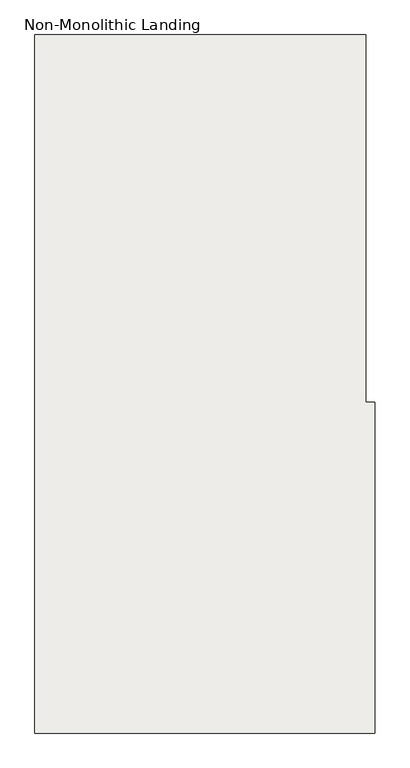
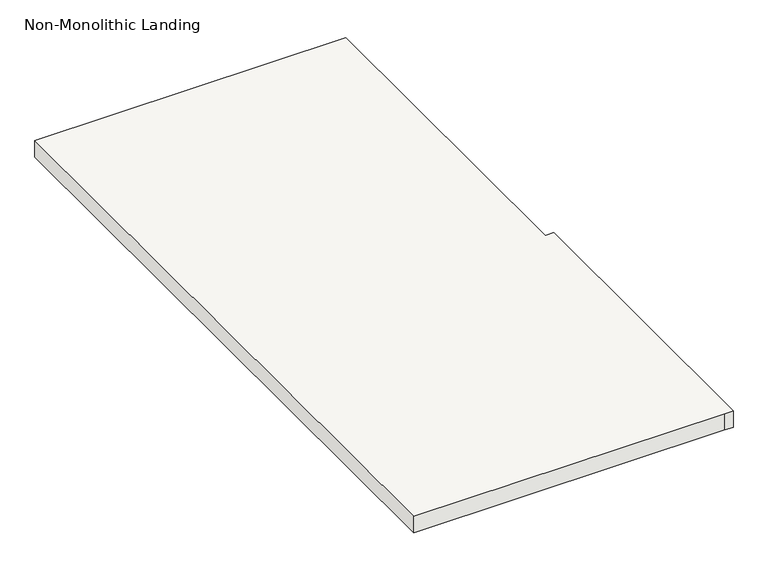
"""IFC4 building model written with IfcOpenShell, lengths in millimetres: slab geometry, Non-Monolithic Landing."""

from ifc_helpers import new_model, si_unit, origin, place, context, project, spatial, faceted_brep, source, transform, mapped, element, save


def non_monolithic_landing_73a33424(model_context):
    return source(origin(), model_context, "Body", "Brep", [
        faceted_brep([(-6394.9112714, -4870.057676, 8001.0), (-6394.9112714, -6800.457676, 8001.0), (-5480.5112714, -6800.457676, 8001.0), (-5455.1112714, -6800.457676, 8001.0), (-5455.1112714, -5886.057676, 8001.0), (-5480.5112714, -5886.057676, 8001.0), (-5480.5112714, -4870.057676, 8001.0), (-5505.9112714, -5784.457676, 7950.2), (-5480.5112714, -5784.457676, 7950.2), (-5480.5112714, -5886.057676, 7950.2), (-5455.1112714, -5886.057676, 7950.2), (-5455.1112714, -6800.457676, 7950.2), (-5480.5112714, -6800.457676, 7950.2), (-6394.9112714, -6800.457676, 7950.2), (-6394.9112714, -4870.057676, 7950.2), (-5505.9112714, -4870.057676, 7950.2), (-5480.5112714, -5784.457676, 7981.95), (-5480.5112714, -4870.057676, 7981.95), (-5505.9112714, -4870.057676, 7956.55), (-5505.9112714, -5784.457676, 7956.55)], [[[0, 1, 2, 3, 4, 5, 6]], [[7, 8, 9, 10, 11, 12, 13, 14, 15]], [[2, 1, 13, 12]], [[4, 3, 11, 10]], [[3, 2, 12, 11]], [[6, 5, 9, 8, 16, 17]], [[0, 6, 17, 18, 15, 14]], [[18, 17, 16, 19]], [[8, 7, 19, 16]], [[7, 15, 18, 19]], [[1, 0, 14, 13]], [[5, 4, 10, 9]]]),
    ])


if __name__ == "__main__":
    model = new_model("IFC4")
    model_context = context("Model", 3, world=origin())
    ifc_project = project(units=[si_unit("LENGTHUNIT", "METRE", prefix="MILLI")], contexts=[model_context])
    site = spatial("IfcSite", under=ifc_project)
    building = spatial("IfcBuilding", under=site)
    placement = place(None, origin())
    non_monolithic_landing_shape = non_monolithic_landing_73a33424(model_context)
    element("IfcSlab", 1, ObjectType="Non-Monolithic Landing", at=placement, inside=building, context=model_context, shape_type="MappedRepresentation", body=[
        mapped(non_monolithic_landing_shape, transform((0.0, 0.0, 0.0), x_axis=(1.0, 0.0, 0.0), y_axis=(0.0, 1.0, 0.0), z_axis=(0.0, 0.0, 1.0))),
    ])
    save(model, "model.ifc")
